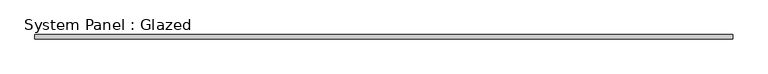
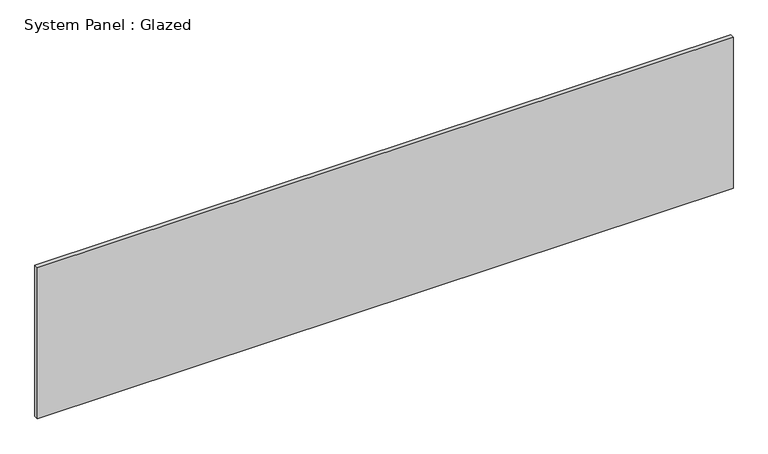
"""IFC4 building model written with IfcOpenShell, lengths in millimetres: plate geometry, System Panel : Glazed."""

from ifc_helpers import new_model, si_unit, origin, origin_with_axes, place, context, project, spatial, polyline, outline, extrude, source, transform, mapped, element, save


def system_panel_glazed_0c970258(model_context):
    return source(origin(), model_context, "Body", "SweptSolid", [
        extrude(outline(polyline([(2089.15, 19.05), (-2089.15, 19.05), (-2089.15, 44.45), (2089.15, 44.45), (2089.15, 19.05)])), origin_with_axes(), (0.0, 0.0, 1.0), 957.9266912),
    ])


if __name__ == "__main__":
    model = new_model("IFC4")
    model_context = context("Model", 3, world=origin())
    ifc_project = project(units=[si_unit("LENGTHUNIT", "METRE", prefix="MILLI")], contexts=[model_context])
    site = spatial("IfcSite", under=ifc_project)
    building = spatial("IfcBuilding", under=site)
    placement = place(None, origin())
    system_panel_glazed_shape = system_panel_glazed_0c970258(model_context)
    element("IfcPlate", 1, ObjectType="System Panel : Glazed", at=placement, inside=building, context=model_context, shape_type="MappedRepresentation", body=[
        mapped(system_panel_glazed_shape, transform((0.0, 0.0, 0.0), x_axis=(1.0, 0.0, 0.0), y_axis=(0.0, 1.0, 0.0), z_axis=(0.0, 0.0, 1.0))),
    ])
    save(model, "model.ifc")

# Revit data of these elements
# Type "System Panel : Glazed"
#   Construction Type Id = "GSP4R"
#   Analytic Construction = "1/8 in Pilkington single glazing"
#   Visual Light Transmittance = 0.9
#   Solar Heat Gain Coefficient = 0.86
#   Heat Transfer Coefficient (U) = 1.18115 BTU/(h·ft²·°F)
#   Define Thermal Properties by = 1
# Element 1 (IfcPlate, "System Panel : Glazed")
#   Materials on its faces: "Glass"
# Materials
#   "Glass": class "Glass", colour RGB 0 128 192, transparency 0.75, Description = "Soda Lime Glass", Cost = 0
